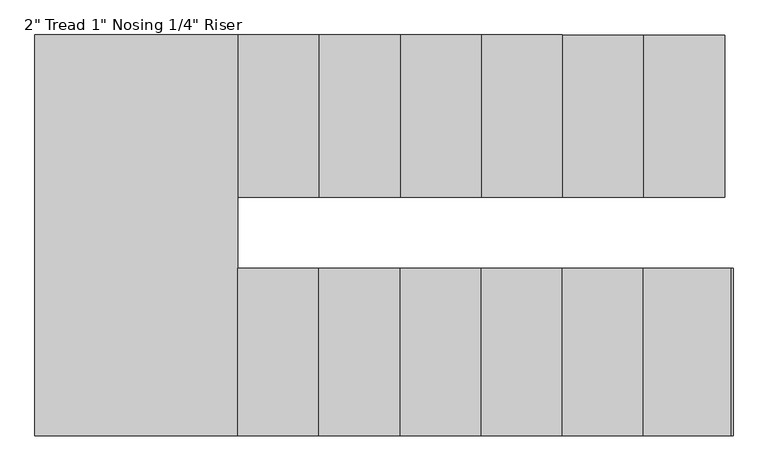
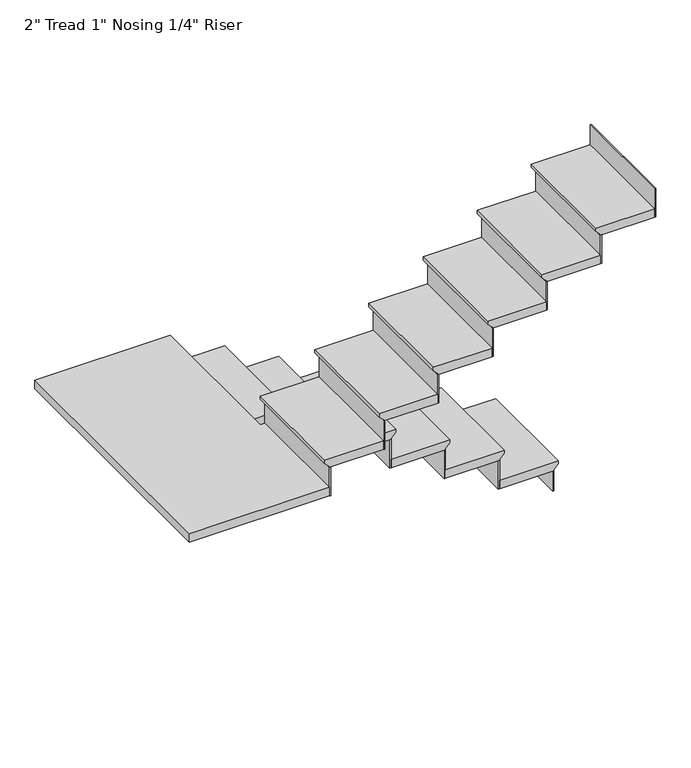
"""IFC4 building model written with IfcOpenShell, lengths in millimetres: stair flight geometry."""

from ifc_helpers import new_model, si_unit, origin, place, context, project, spatial, faceted_brep, source, transform, mapped, element, save


def stair_flight_98403923(model_context):
    return source(origin(), model_context, "Body", "Brep", [
        faceted_brep([(-2968.8120155, -2170.0065691, 9751.4833333), (-2968.8120155, -2170.0065691, 9770.5333333), (-2968.8120155, -2779.6065691, 9770.5333333), (-2968.8120155, -2779.6065691, 9751.4833333), (-2994.2120155, -2170.0065691, 9726.0833333), (-2994.2120155, -2779.6065691, 9726.0833333), (-3299.0120155, -2170.0065691, 9770.5333333), (-3299.0120155, -2779.6065691, 9770.5333333), (-2994.2120155, -2779.6065691, 9719.7333333), (-3299.0120155, -2779.6065691, 9719.7333333), (-3299.0120155, -2170.0065691, 9719.7333333), (-2994.2120155, -2170.0065691, 9719.7333333)], [[[0, 1, 2, 3]], [[4, 0, 3, 5]], [[2, 1, 6, 7]], [[8, 9, 10, 11]], [[2, 7, 9, 8, 5, 3]], [[8, 11, 4, 5]], [[6, 1, 0, 4, 11, 10]], [[7, 6, 10, 9]]]),
        faceted_brep([(-2994.2120155, -2170.0065691, 9719.7333333), (-2994.2120155, -2170.0065691, 9601.2), (-3000.5620155, -2170.0065691, 9601.2), (-3000.5620155, -2170.0065691, 9719.7333333), (-2994.2120155, -2779.6065691, 9719.7333333), (-3000.5620155, -2779.6065691, 9719.7333333), (-3000.5620155, -2779.6065691, 9601.2), (-2994.2120155, -2779.6065691, 9601.2)], [[[0, 1, 2, 3]], [[4, 5, 6, 7]], [[1, 0, 4, 7]], [[2, 1, 7, 6]], [[3, 2, 6, 5]], [[0, 3, 5, 4]]]),
        faceted_brep([(-3299.0120155, -2170.0065691, 9889.0666667), (-3299.0120155, -2170.0065691, 9719.7333333), (-3305.3620155, -2170.0065691, 9719.7333333), (-3305.3620155, -2170.0065691, 9889.0666667), (-3299.0120155, -2779.6065691, 9889.0666667), (-3305.3620155, -2779.6065691, 9889.0666667), (-3305.3620155, -2779.6065691, 9719.7333333), (-3299.0120155, -2779.6065691, 9719.7333333)], [[[0, 1, 2, 3]], [[4, 5, 6, 7]], [[1, 0, 4, 7]], [[2, 1, 7, 6]], [[3, 2, 6, 5]], [[0, 3, 5, 4]]]),
        faceted_brep([(-3273.6120155, -2779.6065691, 9939.8666667), (-3273.6120155, -2170.0065691, 9939.8666667), (-3603.8120155, -2170.0065691, 9939.8666667), (-3603.8120155, -2779.6065691, 9939.8666667), (-3299.0120155, -2779.6065691, 9889.0666667), (-3603.8120155, -2779.6065691, 9889.0666667), (-3603.8120155, -2170.0065691, 9889.0666667), (-3299.0120155, -2170.0065691, 9889.0666667), (-3299.0120155, -2779.6065691, 9895.4166667), (-3273.6120155, -2779.6065691, 9920.8166667), (-3299.0120155, -2170.0065691, 9895.4166667), (-3273.6120155, -2170.0065691, 9920.8166667)], [[[0, 1, 2, 3]], [[4, 5, 6, 7]], [[0, 3, 5, 4, 8, 9]], [[4, 7, 10, 8]], [[2, 1, 11, 10, 7, 6]], [[3, 2, 6, 5]], [[11, 1, 0, 9]], [[10, 11, 9, 8]]]),
        faceted_brep([(-3603.8120155, -2170.0065691, 10058.4), (-3603.8120155, -2170.0065691, 9889.0666667), (-3610.1620155, -2170.0065691, 9889.0666667), (-3610.1620155, -2170.0065691, 10058.4), (-3603.8120155, -2779.6065691, 10058.4), (-3610.1620155, -2779.6065691, 10058.4), (-3610.1620155, -2779.6065691, 9889.0666667), (-3603.8120155, -2779.6065691, 9889.0666667)], [[[0, 1, 2, 3]], [[4, 5, 6, 7]], [[1, 0, 4, 7]], [[2, 1, 7, 6]], [[3, 2, 6, 5]], [[0, 3, 5, 4]]]),
        faceted_brep([(-3578.4120155, -2779.6065691, 10109.2), (-3578.4120155, -2170.0065691, 10109.2), (-3908.6120155, -2170.0065691, 10109.2), (-3908.6120155, -2779.6065691, 10109.2), (-3603.8120155, -2779.6065691, 10058.4), (-3908.6120155, -2779.6065691, 10058.4), (-3908.6120155, -2170.0065691, 10058.4), (-3603.8120155, -2170.0065691, 10058.4), (-3603.8120155, -2779.6065691, 10064.75), (-3578.4120155, -2779.6065691, 10090.15), (-3603.8120155, -2170.0065691, 10064.75), (-3578.4120155, -2170.0065691, 10090.15)], [[[0, 1, 2, 3]], [[4, 5, 6, 7]], [[0, 3, 5, 4, 8, 9]], [[4, 7, 10, 8]], [[2, 1, 11, 10, 7, 6]], [[3, 2, 6, 5]], [[11, 1, 0, 9]], [[10, 11, 9, 8]]]),
        faceted_brep([(-3908.6120155, -2170.0065691, 10227.7333333), (-3908.6120155, -2170.0065691, 10058.4), (-3914.9620155, -2170.0065691, 10058.4), (-3914.9620155, -2170.0065691, 10227.7333333), (-3908.6120155, -2779.6065691, 10227.7333333), (-3914.9620155, -2779.6065691, 10227.7333333), (-3914.9620155, -2779.6065691, 10058.4), (-3908.6120155, -2779.6065691, 10058.4)], [[[0, 1, 2, 3]], [[4, 5, 6, 7]], [[1, 0, 4, 7]], [[2, 1, 7, 6]], [[3, 2, 6, 5]], [[0, 3, 5, 4]]]),
        faceted_brep([(-3883.2120155, -2779.6065691, 10278.5333333), (-3883.2120155, -2170.0065691, 10278.5333333), (-4213.4120155, -2170.0065691, 10278.5333333), (-4213.4120155, -2779.6065691, 10278.5333333), (-3908.6120155, -2779.6065691, 10227.7333333), (-4213.4120155, -2779.6065691, 10227.7333333), (-4213.4120155, -2170.0065691, 10227.7333333), (-3908.6120155, -2170.0065691, 10227.7333333), (-3908.6120155, -2779.6065691, 10234.0833333), (-3883.2120155, -2779.6065691, 10259.4833333), (-3908.6120155, -2170.0065691, 10234.0833333), (-3883.2120155, -2170.0065691, 10259.4833333)], [[[0, 1, 2, 3]], [[4, 5, 6, 7]], [[0, 3, 5, 4, 8, 9]], [[4, 7, 10, 8]], [[2, 1, 11, 10, 7, 6]], [[3, 2, 6, 5]], [[11, 1, 0, 9]], [[10, 11, 9, 8]]]),
        faceted_brep([(-4213.4120155, -2170.0065691, 10397.0666667), (-4213.4120155, -2170.0065691, 10227.7333333), (-4219.7620155, -2170.0065691, 10227.7333333), (-4219.7620155, -2170.0065691, 10397.0666667), (-4213.4120155, -2779.6065691, 10397.0666667), (-4219.7620155, -2779.6065691, 10397.0666667), (-4219.7620155, -2779.6065691, 10227.7333333), (-4213.4120155, -2779.6065691, 10227.7333333)], [[[0, 1, 2, 3]], [[4, 5, 6, 7]], [[1, 0, 4, 7]], [[2, 1, 7, 6]], [[3, 2, 6, 5]], [[0, 3, 5, 4]]]),
        faceted_brep([(-4188.0120155, -2779.6065691, 10447.8666667), (-4188.0120155, -2170.0065691, 10447.8666667), (-4518.2120155, -2170.0065691, 10447.8666667), (-4518.2120155, -2779.6065691, 10447.8666667), (-4213.4120155, -2779.6065691, 10397.0666667), (-4518.2120155, -2779.6065691, 10397.0666667), (-4518.2120155, -2170.0065691, 10397.0666667), (-4213.4120155, -2170.0065691, 10397.0666667), (-4213.4120155, -2779.6065691, 10403.4166667), (-4188.0120155, -2779.6065691, 10428.8166667), (-4213.4120155, -2170.0065691, 10403.4166667), (-4188.0120155, -2170.0065691, 10428.8166667)], [[[0, 1, 2, 3]], [[4, 5, 6, 7]], [[0, 3, 5, 4, 8, 9]], [[4, 7, 10, 8]], [[2, 1, 11, 10, 7, 6]], [[3, 2, 6, 5]], [[11, 1, 0, 9]], [[10, 11, 9, 8]]]),
        faceted_brep([(-4518.2120155, -2170.0065691, 10566.4), (-4518.2120155, -2170.0065691, 10397.0666667), (-4524.5620155, -2170.0065691, 10397.0666667), (-4524.5620155, -2170.0065691, 10566.4), (-4518.2120155, -2779.6065691, 10566.4), (-4524.5620155, -2779.6065691, 10566.4), (-4524.5620155, -2779.6065691, 10397.0666667), (-4518.2120155, -2779.6065691, 10397.0666667)], [[[0, 1, 2, 3]], [[4, 5, 6, 7]], [[1, 0, 4, 7]], [[2, 1, 7, 6]], [[3, 2, 6, 5]], [[0, 3, 5, 4]]]),
        faceted_brep([(-4492.8120155, -2779.6065691, 10617.2), (-4492.8120155, -2170.0065691, 10617.2), (-4823.0120155, -2170.0065691, 10617.2), (-4823.0120155, -2779.6065691, 10617.2), (-4518.2120155, -2779.6065691, 10566.4), (-4823.0120155, -2779.6065691, 10566.4), (-4823.0120155, -2170.0065691, 10566.4), (-4518.2120155, -2170.0065691, 10566.4), (-4518.2120155, -2779.6065691, 10572.75), (-4492.8120155, -2779.6065691, 10598.15), (-4518.2120155, -2170.0065691, 10572.75), (-4492.8120155, -2170.0065691, 10598.15)], [[[0, 1, 2, 3]], [[4, 5, 6, 7]], [[0, 3, 5, 4, 8, 9]], [[4, 7, 10, 8]], [[2, 1, 11, 10, 7, 6]], [[3, 2, 6, 5]], [[11, 1, 0, 9]], [[10, 11, 9, 8]]]),
        faceted_brep([(-4823.0120155, -2170.0065691, 10735.7333333), (-4823.0120155, -2170.0065691, 10566.4), (-4829.3620155, -2170.0065691, 10566.4), (-4829.3620155, -2170.0065691, 10735.7333333), (-4823.0120155, -2779.6065691, 10735.7333333), (-4829.3620155, -2779.6065691, 10735.7333333), (-4829.3620155, -2779.6065691, 10566.4), (-4823.0120155, -2779.6065691, 10566.4)], [[[0, 1, 2, 3]], [[4, 5, 6, 7]], [[1, 0, 4, 7]], [[2, 1, 7, 6]], [[3, 2, 6, 5]], [[0, 3, 5, 4]]]),
        faceted_brep([(-4772.2120155, -3046.3065691, 10786.5333333), (-4797.6120155, -3046.3065691, 10786.5333333), (-4797.6120155, -2170.0065691, 10786.5333333), (-5559.6120155, -2170.0065691, 10786.5333333), (-5559.6120155, -3674.9565691, 10786.5333333), (-4772.2120155, -3674.9565691, 10786.5333333), (-4797.6120155, -3046.3065691, 10735.7333333), (-4772.2120155, -3046.3065691, 10735.7333333), (-4772.2120155, -3674.9565691, 10735.7333333), (-5559.6120155, -3674.9565691, 10735.7333333), (-5559.6120155, -2170.0065691, 10735.7333333), (-4823.0120155, -2170.0065691, 10735.7333333), (-4823.0120155, -2779.6065691, 10735.7333333), (-4797.6120155, -2779.6065691, 10735.7333333), (-4797.6120155, -2779.6065691, 10767.4833333), (-4797.6120155, -2170.0065691, 10767.4833333), (-4823.0120155, -2779.6065691, 10742.0833333), (-4823.0120155, -2170.0065691, 10742.0833333)], [[[0, 1, 2, 3, 4, 5]], [[6, 7, 8, 9, 10, 11, 12, 13]], [[1, 0, 7, 6]], [[2, 1, 6, 13, 14, 15]], [[13, 12, 16, 14]], [[12, 11, 17, 16]], [[3, 2, 15, 17, 11, 10]], [[4, 3, 10, 9]], [[5, 4, 9, 8]], [[0, 5, 8, 7]], [[17, 15, 14, 16]]]),
        faceted_brep([(-4772.2120155, -3674.9565691, 10905.0666667), (-4772.2120155, -3674.9565691, 10735.7333333), (-4765.8620155, -3674.9565691, 10735.7333333), (-4765.8620155, -3674.9565691, 10905.0666667), (-4772.2120155, -3046.3065691, 10905.0666667), (-4765.8620155, -3046.3065691, 10905.0666667), (-4765.8620155, -3046.3065691, 10735.7333333), (-4772.2120155, -3046.3065691, 10735.7333333)], [[[0, 1, 2, 3]], [[4, 5, 6, 7]], [[1, 0, 4, 7]], [[2, 1, 7, 6]], [[3, 2, 6, 5]], [[0, 3, 5, 4]]]),
        faceted_brep([(-4797.6120155, -3046.3065691, 10955.8666667), (-4797.6120155, -3674.9565691, 10955.8666667), (-4467.4120155, -3674.9565691, 10955.8666667), (-4467.4120155, -3046.3065691, 10955.8666667), (-4772.2120155, -3046.3065691, 10905.0666667), (-4467.4120155, -3046.3065691, 10905.0666667), (-4467.4120155, -3674.9565691, 10905.0666667), (-4772.2120155, -3674.9565691, 10905.0666667), (-4772.2120155, -3046.3065691, 10911.4166667), (-4797.6120155, -3046.3065691, 10936.8166667), (-4772.2120155, -3674.9565691, 10911.4166667), (-4797.6120155, -3674.9565691, 10936.8166667)], [[[0, 1, 2, 3]], [[4, 5, 6, 7]], [[0, 3, 5, 4, 8, 9]], [[4, 7, 10, 8]], [[2, 1, 11, 10, 7, 6]], [[3, 2, 6, 5]], [[11, 1, 0, 9]], [[10, 11, 9, 8]]]),
        faceted_brep([(-4467.4120155, -3674.9565691, 11074.4), (-4467.4120155, -3674.9565691, 10905.0666667), (-4461.0620155, -3674.9565691, 10905.0666667), (-4461.0620155, -3674.9565691, 11074.4), (-4467.4120155, -3046.3065691, 11074.4), (-4461.0620155, -3046.3065691, 11074.4), (-4461.0620155, -3046.3065691, 10905.0666667), (-4467.4120155, -3046.3065691, 10905.0666667)], [[[0, 1, 2, 3]], [[4, 5, 6, 7]], [[1, 0, 4, 7]], [[2, 1, 7, 6]], [[3, 2, 6, 5]], [[0, 3, 5, 4]]]),
        faceted_brep([(-4492.8120155, -3046.3065691, 11125.2), (-4492.8120155, -3674.9565691, 11125.2), (-4162.6120155, -3674.9565691, 11125.2), (-4162.6120155, -3046.3065691, 11125.2), (-4467.4120155, -3046.3065691, 11074.4), (-4162.6120155, -3046.3065691, 11074.4), (-4162.6120155, -3674.9565691, 11074.4), (-4467.4120155, -3674.9565691, 11074.4), (-4467.4120155, -3046.3065691, 11080.75), (-4492.8120155, -3046.3065691, 11106.15), (-4467.4120155, -3674.9565691, 11080.75), (-4492.8120155, -3674.9565691, 11106.15)], [[[0, 1, 2, 3]], [[4, 5, 6, 7]], [[0, 3, 5, 4, 8, 9]], [[4, 7, 10, 8]], [[2, 1, 11, 10, 7, 6]], [[3, 2, 6, 5]], [[11, 1, 0, 9]], [[10, 11, 9, 8]]]),
        faceted_brep([(-4162.6120155, -3674.9565691, 11243.7333333), (-4162.6120155, -3674.9565691, 11074.4), (-4156.2620155, -3674.9565691, 11074.4), (-4156.2620155, -3674.9565691, 11243.7333333), (-4162.6120155, -3046.3065691, 11243.7333333), (-4156.2620155, -3046.3065691, 11243.7333333), (-4156.2620155, -3046.3065691, 11074.4), (-4162.6120155, -3046.3065691, 11074.4)], [[[0, 1, 2, 3]], [[4, 5, 6, 7]], [[1, 0, 4, 7]], [[2, 1, 7, 6]], [[3, 2, 6, 5]], [[0, 3, 5, 4]]]),
        faceted_brep([(-4188.0120155, -3046.3065691, 11294.5333333), (-4188.0120155, -3674.9565691, 11294.5333333), (-3857.8120155, -3674.9565691, 11294.5333333), (-3857.8120155, -3046.3065691, 11294.5333333), (-4162.6120155, -3046.3065691, 11243.7333333), (-3857.8120155, -3046.3065691, 11243.7333333), (-3857.8120155, -3674.9565691, 11243.7333333), (-4162.6120155, -3674.9565691, 11243.7333333), (-4162.6120155, -3046.3065691, 11250.0833333), (-4188.0120155, -3046.3065691, 11275.4833333), (-4162.6120155, -3674.9565691, 11250.0833333), (-4188.0120155, -3674.9565691, 11275.4833333)], [[[0, 1, 2, 3]], [[4, 5, 6, 7]], [[0, 3, 5, 4, 8, 9]], [[4, 7, 10, 8]], [[2, 1, 11, 10, 7, 6]], [[3, 2, 6, 5]], [[11, 1, 0, 9]], [[10, 11, 9, 8]]]),
        faceted_brep([(-3857.8120155, -3674.9565691, 11413.0666667), (-3857.8120155, -3674.9565691, 11243.7333333), (-3851.4620155, -3674.9565691, 11243.7333333), (-3851.4620155, -3674.9565691, 11413.0666667), (-3857.8120155, -3046.3065691, 11413.0666667), (-3851.4620155, -3046.3065691, 11413.0666667), (-3851.4620155, -3046.3065691, 11243.7333333), (-3857.8120155, -3046.3065691, 11243.7333333)], [[[0, 1, 2, 3]], [[4, 5, 6, 7]], [[1, 0, 4, 7]], [[2, 1, 7, 6]], [[3, 2, 6, 5]], [[0, 3, 5, 4]]]),
        faceted_brep([(-3883.2120155, -3046.3065691, 11463.8666667), (-3883.2120155, -3674.9565691, 11463.8666667), (-3553.0120155, -3674.9565691, 11463.8666667), (-3553.0120155, -3046.3065691, 11463.8666667), (-3857.8120155, -3046.3065691, 11413.0666667), (-3553.0120155, -3046.3065691, 11413.0666667), (-3553.0120155, -3674.9565691, 11413.0666667), (-3857.8120155, -3674.9565691, 11413.0666667), (-3857.8120155, -3046.3065691, 11419.4166667), (-3883.2120155, -3046.3065691, 11444.8166667), (-3857.8120155, -3674.9565691, 11419.4166667), (-3883.2120155, -3674.9565691, 11444.8166667)], [[[0, 1, 2, 3]], [[4, 5, 6, 7]], [[0, 3, 5, 4, 8, 9]], [[4, 7, 10, 8]], [[2, 1, 11, 10, 7, 6]], [[3, 2, 6, 5]], [[11, 1, 0, 9]], [[10, 11, 9, 8]]]),
        faceted_brep([(-3553.0120155, -3674.9565691, 11582.4), (-3553.0120155, -3674.9565691, 11413.0666667), (-3546.6620155, -3674.9565691, 11413.0666667), (-3546.6620155, -3674.9565691, 11582.4), (-3553.0120155, -3046.3065691, 11582.4), (-3546.6620155, -3046.3065691, 11582.4), (-3546.6620155, -3046.3065691, 11413.0666667), (-3553.0120155, -3046.3065691, 11413.0666667)], [[[0, 1, 2, 3]], [[4, 5, 6, 7]], [[1, 0, 4, 7]], [[2, 1, 7, 6]], [[3, 2, 6, 5]], [[0, 3, 5, 4]]]),
        faceted_brep([(-3578.4120155, -3046.3065691, 11633.2), (-3578.4120155, -3674.9565691, 11633.2), (-3248.2120155, -3674.9565691, 11633.2), (-3248.2120155, -3046.3065691, 11633.2), (-3553.0120155, -3046.3065691, 11582.4), (-3248.2120155, -3046.3065691, 11582.4), (-3248.2120155, -3674.9565691, 11582.4), (-3553.0120155, -3674.9565691, 11582.4), (-3553.0120155, -3046.3065691, 11588.75), (-3578.4120155, -3046.3065691, 11614.15), (-3553.0120155, -3674.9565691, 11588.75), (-3578.4120155, -3674.9565691, 11614.15)], [[[0, 1, 2, 3]], [[4, 5, 6, 7]], [[0, 3, 5, 4, 8, 9]], [[4, 7, 10, 8]], [[2, 1, 11, 10, 7, 6]], [[3, 2, 6, 5]], [[11, 1, 0, 9]], [[10, 11, 9, 8]]]),
        faceted_brep([(-3248.2120155, -3674.9565691, 11751.7333333), (-3248.2120155, -3674.9565691, 11582.4), (-3241.8620155, -3674.9565691, 11582.4), (-3241.8620155, -3674.9565691, 11751.7333333), (-3248.2120155, -3046.3065691, 11751.7333333), (-3241.8620155, -3046.3065691, 11751.7333333), (-3241.8620155, -3046.3065691, 11582.4), (-3248.2120155, -3046.3065691, 11582.4)], [[[0, 1, 2, 3]], [[4, 5, 6, 7]], [[1, 0, 4, 7]], [[2, 1, 7, 6]], [[3, 2, 6, 5]], [[0, 3, 5, 4]]]),
        faceted_brep([(-2943.4120155, -3674.9565691, 11921.0666667), (-2943.4120155, -3674.9565691, 11751.7333333), (-2937.0620155, -3674.9565691, 11751.7333333), (-2937.0620155, -3674.9565691, 11921.0666667), (-2943.4120155, -3046.3065691, 11921.0666667), (-2937.0620155, -3046.3065691, 11921.0666667), (-2937.0620155, -3046.3065691, 11751.7333333), (-2943.4120155, -3046.3065691, 11751.7333333)], [[[0, 1, 2, 3]], [[4, 5, 6, 7]], [[1, 0, 4, 7]], [[2, 1, 7, 6]], [[3, 2, 6, 5]], [[0, 3, 5, 4]]]),
        faceted_brep([(-3273.6120155, -3046.3065691, 11802.5333333), (-3273.6120155, -3674.9565691, 11802.5333333), (-2943.4120155, -3674.9565691, 11802.5333333), (-2943.4120155, -3046.3065691, 11802.5333333), (-3248.2120155, -3046.3065691, 11751.7333333), (-2943.4120155, -3046.3065691, 11751.7333333), (-2943.4120155, -3674.9565691, 11751.7333333), (-3248.2120155, -3674.9565691, 11751.7333333), (-3248.2120155, -3046.3065691, 11758.0833333), (-3273.6120155, -3046.3065691, 11783.4833333), (-3248.2120155, -3674.9565691, 11758.0833333), (-3273.6120155, -3674.9565691, 11783.4833333)], [[[0, 1, 2, 3]], [[4, 5, 6, 7]], [[0, 3, 5, 4, 8, 9]], [[4, 7, 10, 8]], [[2, 1, 11, 10, 7, 6]], [[3, 2, 6, 5]], [[11, 1, 0, 9]], [[10, 11, 9, 8]]]),
    ])


if __name__ == "__main__":
    model = new_model("IFC4")
    model_context = context("Model", 3, world=origin())
    ifc_project = project(units=[si_unit("LENGTHUNIT", "METRE", prefix="MILLI")], contexts=[model_context])
    site = spatial("IfcSite", under=ifc_project)
    building = spatial("IfcBuilding", under=site)
    placement = place(None, origin())
    stair_flight_shape = stair_flight_98403923(model_context)
    element("IfcStairFlight", 1, ObjectType="2\" Tread 1\" Nosing 1/4\" Riser", at=placement, inside=building, context=model_context, shape_type="MappedRepresentation", body=[
        mapped(stair_flight_shape, transform((0.0, 0.0, 0.0), x_axis=(1.0, 0.0, 0.0), y_axis=(0.0, 1.0, 0.0), z_axis=(0.0, 0.0, 1.0))),
    ])
    save(model, "model.ifc")
